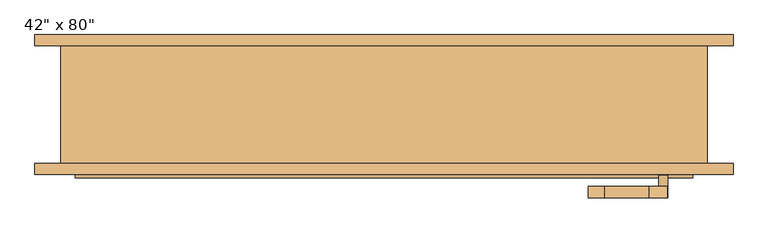
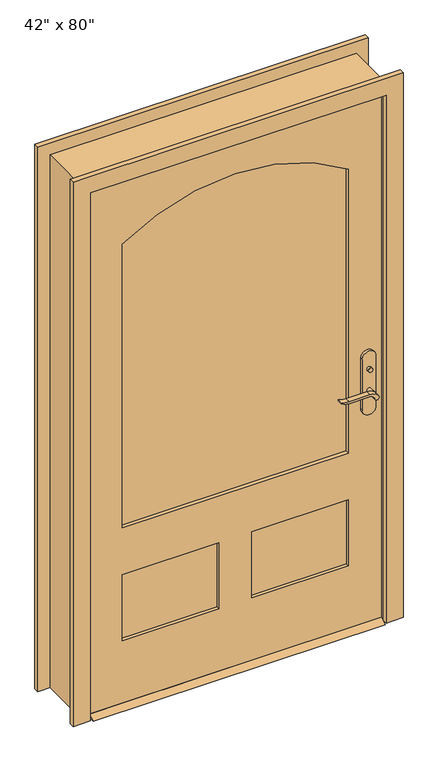
"""IFC4 building model written with IfcOpenShell, lengths in millimetres: door geometry."""

from ifc_helpers import new_model, si_unit, point, frame, frame_2d, origin, place, context, project, spatial, polyline, circle_curve, trimmed, segment, composite_curve, outline, extrude, faceted_brep, source, transform, mapped, element, save


def door_fa6f8c62(model_context):
    return source(origin(), model_context, "Body", "SolidModel", [
        extrude(outline(polyline([(-63.5, 12.7), (-38.1, 0.0), (-123.825, 0.0), (-98.425, 12.7), (-63.5, 12.7)])), frame((-533.4, 0.0, 0.0), z_axis=(1.0, 0.0, 0.0), x_axis=(0.0, 1.0, 0.0)), (0.0, 0.0, 1.0), 1066.8),
        extrude(outline(polyline([(487.6, -43.5), (487.6, -53.5), (477.6, -53.5), (477.6, -43.5), (487.6, -43.5)])), frame((0.0, 0.0, 981.9), z_axis=(0.0, 0.0, 1.0), x_axis=(1.0, 0.0, 0.0)), (0.0, 0.0, 1.0), 30.0),
        extrude(outline(composite_curve([segment(trimmed(circle_curve(frame_2d((996.9, 482.6)), 8.0), [point((996.9, 474.6))], [point((996.9, 490.6))], False, "CARTESIAN"), True, "CONTINUOUS"), segment(trimmed(circle_curve(frame_2d((996.9, 482.6)), 8.0), [point((996.9, 490.6))], [point((996.9, 474.6))], False, "CARTESIAN"), True, "CONTINUOUS")], self_intersect=False)), frame((0.0, -118.425, 0.0), z_axis=(0.0, 1.0, 0.0), x_axis=(0.0, 0.0, 1.0)), (0.0, 0.0, 1.0), 10.0),
        extrude(outline(composite_curve([segment(trimmed(circle_curve(frame_2d((897.1555521, 458.9324871)), 37.2832219), [point((919.0523287, 489.1081363))], [point((934.4, 457.2325667))], False, "CARTESIAN"), True, "CONTINUOUS"), segment(polyline([(934.4, 457.2325667), (934.4, 380.9564091)]), True, "CONTINUOUS"), segment(trimmed(circle_curve(frame_2d((1017.6850638, 381.0227909)), 83.2850902), [point((934.4, 380.9564091))], [point((939.4, 352.6))], True, "CARTESIAN"), True, "CONTINUOUS"), segment(polyline([(939.4, 352.6), (936.6135558, 352.6)]), True, "CONTINUOUS"), segment(trimmed(circle_curve(frame_2d((986.6709207, 384.5396612)), 59.3791355), [point((936.6135558, 352.6))], [point((927.4, 380.9564091))], False, "CARTESIAN"), True, "CONTINUOUS"), segment(polyline([(927.4, 380.9564091), (927.4, 457.2138099)]), True, "CONTINUOUS"), segment(trimmed(circle_curve(frame_2d((909.2738613, 457.2138099)), 18.1261387), [point((927.4, 457.2138099))], [point((914.4, 474.6))], True, "CARTESIAN"), True, "CONTINUOUS"), segment(trimmed(circle_curve(frame_2d((914.4, 482.6)), 8.0), [point((914.4, 474.6))], [point((919.0523287, 489.1081363))], False, "CARTESIAN"), True, "CONTINUOUS")], self_intersect=False)), frame((0.0, -23.5, 0.0), z_axis=(0.0, 1.0, 0.0), x_axis=(0.0, 0.0, 1.0)), (0.0, 0.0, 1.0), 20.0),
        extrude(outline(composite_curve([segment(trimmed(circle_curve(frame_2d((914.4, 482.6)), 8.0), [point((914.3999903, 474.6))], [point((919.0523287, 489.1081363))], False, "CARTESIAN"), True, "CONTINUOUS"), segment(trimmed(circle_curve(frame_2d((897.1555521, 458.9324871)), 37.2832219), [point((919.0523287, 489.1081363))], [point((934.4, 457.2325667))], False, "CARTESIAN"), True, "CONTINUOUS"), segment(polyline([(934.4, 457.2325667), (934.4, 380.9564091)]), True, "CONTINUOUS"), segment(trimmed(circle_curve(frame_2d((1017.6850638, 381.0227909)), 83.2850902), [point((934.4, 380.9564091))], [point((939.4, 352.6))], True, "CARTESIAN"), True, "CONTINUOUS"), segment(polyline([(939.4, 352.6), (936.6135558, 352.6)]), True, "CONTINUOUS"), segment(trimmed(circle_curve(frame_2d((986.6709207, 384.5396612)), 59.3791355), [point((936.6135558, 352.6))], [point((927.4, 380.9564091))], False, "CARTESIAN"), True, "CONTINUOUS"), segment(polyline([(927.4, 380.9564091), (927.4, 457.2138122)]), True, "CONTINUOUS"), segment(trimmed(circle_curve(frame_2d((909.2738682, 457.2138122)), 18.1261318), [point((927.4, 457.2138122))], [point((914.3999903, 474.6))], True, "CARTESIAN"), True, "CONTINUOUS")], self_intersect=False)), frame((0.0, -158.425, 0.0), z_axis=(0.0, 1.0, 0.0), x_axis=(0.0, 0.0, 1.0)), (0.0, 0.0, 1.0), 20.0),
        extrude(outline(composite_curve([segment(trimmed(circle_curve(frame_2d((914.4, 482.6)), 8.0), [point((914.4, 474.6))], [point((914.4, 490.6))], False, "CARTESIAN"), True, "CONTINUOUS"), segment(trimmed(circle_curve(frame_2d((914.4, 482.6)), 8.0), [point((914.4, 490.6))], [point((914.4, 474.6))], False, "CARTESIAN"), True, "CONTINUOUS")], self_intersect=False)), frame((0.0, -53.5, 0.0), z_axis=(0.0, 1.0, 0.0), x_axis=(0.0, 0.0, 1.0)), (0.0, 0.0, 1.0), 30.0),
        extrude(outline(composite_curve([segment(trimmed(circle_curve(frame_2d((914.4, 482.6)), 8.0), [point((914.4, 474.6))], [point((914.4, 490.6))], False, "CARTESIAN"), True, "CONTINUOUS"), segment(trimmed(circle_curve(frame_2d((914.4, 482.6)), 8.0), [point((914.4, 490.6))], [point((914.4, 474.6))], False, "CARTESIAN"), True, "CONTINUOUS")], self_intersect=False)), frame((0.0, -138.425, 0.0), z_axis=(0.0, 1.0, 0.0), x_axis=(0.0, 0.0, 1.0)), (0.0, 0.0, 1.0), 30.0),
        extrude(outline(composite_curve([segment(polyline([(844.4, 507.6), (1039.4, 507.6)]), True, "CONTINUOUS"), segment(trimmed(circle_curve(frame_2d((1039.4, 482.6)), 25.0), [point((1039.4, 507.6))], [point((1039.4, 457.6))], False, "CARTESIAN"), True, "CONTINUOUS"), segment(polyline([(1039.4, 457.6), (844.4, 457.6)]), True, "CONTINUOUS"), segment(trimmed(circle_curve(frame_2d((844.4, 482.6)), 25.0), [point((844.4, 457.6))], [point((844.4, 507.6))], False, "CARTESIAN"), True, "CONTINUOUS")], self_intersect=False)), frame((0.0, -63.5, 0.0), z_axis=(0.0, 1.0, 0.0), x_axis=(0.0, 0.0, 1.0)), (0.0, 0.0, 1.0), 10.0),
        extrude(outline(composite_curve([segment(polyline([(844.4, 507.6), (1039.4, 507.6)]), True, "CONTINUOUS"), segment(trimmed(circle_curve(frame_2d((1039.4, 482.6)), 25.0), [point((1039.4, 507.6))], [point((1039.4, 457.6))], False, "CARTESIAN"), True, "CONTINUOUS"), segment(polyline([(1039.4, 457.6), (844.4, 457.6)]), True, "CONTINUOUS"), segment(trimmed(circle_curve(frame_2d((844.4, 482.6)), 25.0), [point((844.4, 457.6))], [point((844.4, 507.6))], False, "CARTESIAN"), True, "CONTINUOUS")], self_intersect=False)), frame((0.0, -108.425, 0.0), z_axis=(0.0, 1.0, 0.0), x_axis=(0.0, 0.0, 1.0)), (0.0, 0.0, 1.0), 10.0),
        extrude(outline(polyline([(2032.0, -533.4), (12.7, -533.4), (12.7, 533.4), (2032.0, 533.4), (2032.0, -533.4)]), holes=[composite_curve([segment(polyline([(688.975, -412.75), (1784.35, -412.75)]), True, "CONTINUOUS"), segment(trimmed(circle_curve(frame_2d((1177.13125, 0.0)), 734.21875), [point((1784.35, -412.75))], [point((1784.35, 412.75))], True, "CARTESIAN"), True, "CONTINUOUS"), segment(polyline([(1784.35, 412.75), (688.975, 412.75), (688.975, -412.75)]), True, "CONTINUOUS")], self_intersect=False), polyline([(508.0, -60.325), (254.0, -60.325), (254.0, -412.75), (508.0, -412.75), (508.0, -60.325)]), polyline([(508.0, 412.75), (254.0, 412.75), (254.0, 60.325), (508.0, 60.325), (508.0, 412.75)])]), frame((0.0, -98.425, 0.0), z_axis=(0.0, 1.0, 0.0), x_axis=(0.0, 0.0, 1.0)), (0.0, 0.0, 1.0), 34.925),
        faceted_brep([(558.8, -98.425, 0.0), (533.4, -98.425, 0.0), (533.4, -63.5, 0.0), (520.7, -63.5, 0.0), (520.7, -28.575, 0.0), (533.4, -28.575, 0.0), (533.4, 104.775, 0.0), (558.8, 104.775, 0.0), (558.8, 104.775, 2057.4), (558.8, -98.425, 2057.4), (533.4, 104.775, 2032.0), (-533.4, 104.775, 2032.0), (-533.4, 104.775, 0.0), (-558.8, 104.775, 0.0), (-558.8, 104.775, 2057.4), (533.4, -28.575, 2032.0), (520.7, -28.575, 2019.3), (-520.7, -28.575, 2019.3), (-520.7, -28.575, 0.0), (-533.4, -28.575, 0.0), (-533.4, -28.575, 2032.0), (520.7, -63.5, 2019.3), (533.4, -63.5, 2032.0), (-533.4, -63.5, 2032.0), (-533.4, -63.5, 0.0), (-520.7, -63.5, 0.0), (-520.7, -63.5, 2019.3), (533.4, -98.425, 2032.0), (-558.8, -98.425, 2057.4), (-558.8, -98.425, 0.0), (-533.4, -98.425, 0.0), (-533.4, -98.425, 2032.0)], [[[0, 1, 2, 3, 4, 5, 6, 7]], [[7, 8, 9, 0]], [[6, 10, 11, 12, 13, 14, 8, 7]], [[5, 15, 10, 6]], [[4, 16, 17, 18, 19, 20, 15, 5]], [[3, 21, 16, 4]], [[2, 22, 23, 24, 25, 26, 21, 3]], [[1, 27, 22, 2]], [[0, 9, 28, 29, 30, 31, 27, 1]], [[8, 14, 28, 9]], [[15, 20, 11, 10]], [[21, 26, 17, 16]], [[27, 31, 23, 22]], [[29, 13, 12, 19, 18, 25, 24, 30]], [[14, 13, 29, 28]], [[20, 19, 12, 11]], [[26, 25, 18, 17]], [[31, 30, 24, 23]]]),
        extrude(outline(polyline([(-60.325, -75.1416667), (-60.325, -86.7833333), (-412.75, -86.7833333), (-412.75, -75.1416667), (-60.325, -75.1416667)])), frame((0.0, 0.0, 254.0), z_axis=(0.0, 0.0, 1.0), x_axis=(1.0, 0.0, 0.0)), (0.0, 0.0, 1.0), 254.0),
        extrude(outline(polyline([(412.75, -75.1416667), (412.75, -86.7833333), (60.325, -86.7833333), (60.325, -75.1416667), (412.75, -75.1416667)])), frame((0.0, 0.0, 254.0), z_axis=(0.0, 0.0, 1.0), x_axis=(1.0, 0.0, 0.0)), (0.0, 0.0, 1.0), 254.0),
        extrude(outline(composite_curve([segment(polyline([(688.975, -412.75), (688.975, 412.75), (1784.35, 412.75)]), True, "CONTINUOUS"), segment(trimmed(circle_curve(frame_2d((1177.13125, 0.0)), 734.21875), [point((1784.35, 412.75))], [point((1784.35, -412.75))], False, "CARTESIAN"), True, "CONTINUOUS"), segment(polyline([(1784.35, -412.75), (688.975, -412.75)]), True, "CONTINUOUS")], self_intersect=False)), frame((0.0, -84.455, 0.0), z_axis=(0.0, 1.0, 0.0), x_axis=(0.0, 0.0, 1.0)), (0.0, 0.0, 1.0), 6.985),
        extrude(outline(polyline([(0.0, -539.75), (2038.35, -539.75), (2038.35, 539.75), (0.0, 539.75), (0.0, 603.25), (2101.85, 603.25), (2101.85, -603.25), (0.0, -603.25), (0.0, -539.75)])), frame((0.0, 104.775, 0.0), z_axis=(0.0, 1.0, 0.0), x_axis=(0.0, 0.0, 1.0)), (0.0, 0.0, 1.0), 19.05),
        extrude(outline(polyline([(0.0, -539.75), (2038.35, -539.75), (2038.35, 539.75), (0.0, 539.75), (0.0, 603.25), (2101.85, 603.25), (2101.85, -603.25), (0.0, -603.25), (0.0, -539.75)])), frame((0.0, -117.475, 0.0), z_axis=(0.0, 1.0, 0.0), x_axis=(0.0, 0.0, 1.0)), (0.0, 0.0, 1.0), 19.05),
    ])


if __name__ == "__main__":
    model = new_model("IFC4")
    model_context = context("Model", 3, world=origin())
    ifc_project = project(units=[si_unit("LENGTHUNIT", "METRE", prefix="MILLI")], contexts=[model_context])
    site = spatial("IfcSite", under=ifc_project)
    building = spatial("IfcBuilding", under=site)
    placement = place(None, origin())
    door_shape = door_fa6f8c62(model_context)
    element("IfcDoor", 1, ObjectType="42\" x 80\"", at=placement, inside=building, context=model_context, shape_type="MappedRepresentation", body=[
        mapped(door_shape, transform((0.0, 0.0, 0.0), x_axis=(1.0, 0.0, 0.0), y_axis=(0.0, 1.0, 0.0), z_axis=(0.0, 0.0, 1.0))),
    ])
    save(model, "model.ifc")

# Revit data of these elements
# Type "42\" x 80\""
#   Type Mark = "9"
#   Assembly Code = "B2030100"
#   Analytic Construction = "French door, wood frame with single glass"
#   Threshold Offset [instance default] = 0' - 0 1/2"
#   Thickness = 0' - 1 3/8"
#   Thermal Resistance (R) = 1.0696 (h·ft²·°F)/BTU
#   Swing Angle [instance default] = 90.00°
#   Stiles = 0' - 4 3/4"
#   Rough Width = 3' - 8"
#   Rough Height = 6' - 9"
#   Radius = 2' - 4 29/32"
#   Lock Rail = 0' - 7 1/8"
#   Height = 6' - 8"
#   Width = 3' - 6"
#   Heat Transfer Coefficient (U) = 0.9350 BTU/(h·ft²·°F)
#   Door Offset [instance default] = 0' - 0"
#   Bottom Rail = 0' - 9 1/2"
#   Threshold [instance default] = yes
#   Function = 1
#   Exterior Trim [instance default] = yes
#   Trim Material = Cherry
#   Threshold Material = Cherry
#   Panel Material = Cherry
#   Glazing = Glass
#   Frame Material = Cherry
#   Door Handle Material = Aluminum
#   Visual Light Transmittance = 0
#   Solar Heat Gain Coefficient = 0
#   Wall Closure = (empty or 0)
#   Construction Type = (empty or 0)
# Element 1 (IfcDoor, "42\" x 80\"")
#   Materials on its faces: "Cherry", "Aluminum", "Glass"
# Materials
#   "Cherry": class "Wood", colour RGB 226 177 128, transparency 0, Description = "Prunus Serotina", Cost = 0
#   "Glass": class "Glass", colour RGB 0 128 192, transparency 0.75, Description = "Soda Lime Glass", Cost = 0
#   "Aluminum": class "Metal", colour RGB 247 247 247, transparency 0, Description = "Aluminum 6061", Cost = 0
